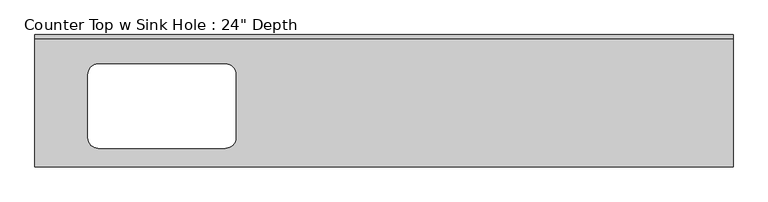
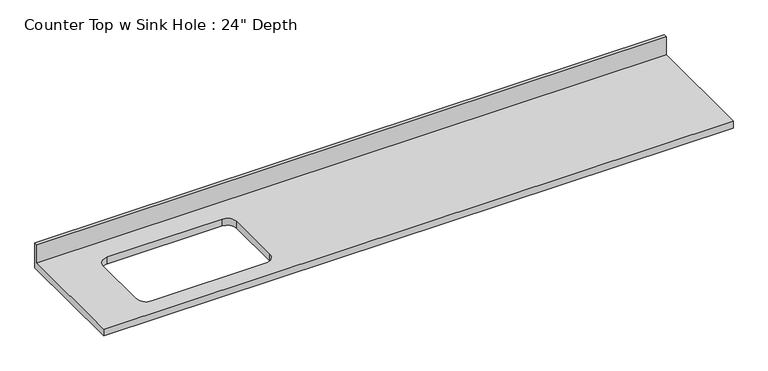
"""IFC4 building model written with IfcOpenShell, lengths in millimetres: furniture geometry."""

from ifc_helpers import new_model, si_unit, frame, origin, place, context, project, spatial, polyline, circle_curve, source, transform, mapped, element, save
from ifc_brep_helpers import plane_surface, revolved_surface, advanced_brep


def furniture_691b2c5f(model_context):
    return source(origin(), model_context, "Body", "AdvancedBrep", [
        advanced_brep(
        [(-1200.4622951, -635.0, 914.4), (2152.3377049, -635.0, 914.4), (2152.3377049, -19.05, 914.4), (-1200.4622951, -19.05, 914.4), (-895.6622951, -139.7, 914.4), (-286.0622951, -139.7, 914.4), (-235.2622951, -190.5, 914.4), (-235.2622951, -495.3, 914.4), (-286.0622951, -546.1, 914.4), (-895.6622951, -546.1, 914.4), (-946.4622951, -495.3, 914.4), (-946.4622951, -190.5, 914.4), (2152.3377049, 0.0, 876.3), (2152.3377049, -635.0, 876.3), (-1200.4622951, -635.0, 876.3), (-1200.4622951, 0.0, 876.3), (-286.0622951, -139.7, 876.3), (-895.6622951, -139.7, 876.3), (-946.4622951, -190.5, 876.3), (-946.4622951, -495.3, 876.3), (-895.6622951, -546.1, 876.3), (-286.0622951, -546.1, 876.3), (-235.2622951, -495.3, 876.3), (-235.2622951, -190.5, 876.3), (-1200.4622951, 0.0, 1016.0), (2152.3377049, 0.0, 1016.0), (-1200.4622951, -19.05, 1016.0), (2152.3377049, -19.05, 1016.0)],
        [
            (0, 1),
            (1, 2),
            (2, 3),
            (3, 0),
            (4, 5),
            (5, 6, circle_curve(frame((-286.0622951, -190.5, 914.4), z_axis=(0.0, 0.0, -1.0), x_axis=(1.0, 0.0, 0.0)), 50.8)),
            (6, 7),
            (7, 8, circle_curve(frame((-286.0622951, -495.3, 914.4), z_axis=(0.0, 0.0, -1.0), x_axis=(1.0, 0.0, 0.0)), 50.8)),
            (8, 9),
            (9, 10, circle_curve(frame((-895.6622951, -495.3, 914.4), z_axis=(0.0, 0.0, -1.0), x_axis=(1.0, 0.0, 0.0)), 50.8)),
            (10, 11),
            (11, 4, circle_curve(frame((-895.6622951, -190.5, 914.4), z_axis=(0.0, 0.0, -1.0), x_axis=(1.0, 0.0, 0.0)), 50.8)),
            (12, 13),
            (13, 14),
            (14, 15),
            (15, 12),
            (16, 17),
            (17, 18, circle_curve(frame((-895.6622951, -190.5, 876.3), z_axis=(0.0, 0.0, 1.0), x_axis=(1.0, 0.0, 0.0)), 50.8)),
            (18, 19),
            (19, 20, circle_curve(frame((-895.6622951, -495.3, 876.3), z_axis=(0.0, 0.0, 1.0), x_axis=(1.0, 0.0, 0.0)), 50.8)),
            (20, 21),
            (21, 22, circle_curve(frame((-286.0622951, -495.3, 876.3), z_axis=(0.0, 0.0, 1.0), x_axis=(1.0, 0.0, 0.0)), 50.8)),
            (22, 23),
            (23, 16, circle_curve(frame((-286.0622951, -190.5, 876.3), z_axis=(0.0, 0.0, 1.0), x_axis=(1.0, 0.0, 0.0)), 50.8)),
            (15, 24),
            (24, 25),
            (25, 12),
            (14, 0),
            (3, 26),
            (26, 24),
            (13, 1),
            (25, 27),
            (27, 2),
            (26, 27),
            (4, 17),
            (16, 5),
            (11, 18),
            (10, 19),
            (9, 20),
            (8, 21),
            (7, 22),
            (6, 23),
        ],
        [
            plane_surface(frame((-1200.4622951, 0.0, 914.4), z_axis=(0.0, 0.0, 1.0), x_axis=(-1.0, 0.0, 0.0))),
            plane_surface(frame((-1200.4622951, 0.0, 876.3), z_axis=(0.0, 0.0, -1.0), x_axis=(1.0, 0.0, 0.0))),
            plane_surface(frame((2152.3377049, 0.0, 914.4), z_axis=(0.0, 1.0, 0.0), x_axis=(0.0, 0.0, -1.0))),
            plane_surface(frame((-1200.4622951, 0.0, 914.4), z_axis=(-1.0, 0.0, 0.0), x_axis=(0.0, 0.0, -1.0))),
            plane_surface(frame((-1200.4622951, -635.0, 914.4), z_axis=(0.0, -1.0, 0.0), x_axis=(0.0, 0.0, -1.0))),
            plane_surface(frame((2152.3377049, -635.0, 914.4), z_axis=(1.0, 0.0, 0.0), x_axis=(0.0, 0.0, -1.0))),
            plane_surface(frame((-1200.4622951, 0.0, 1016.0), z_axis=(0.0, 0.0, 1.0), x_axis=(0.0, -1.0, 0.0))),
            plane_surface(frame((-1200.4622951, -19.05, 1016.0), z_axis=(0.0, -1.0, 0.0), x_axis=(0.0, 0.0, -1.0))),
            plane_surface(frame((-286.0622951, -139.7, 914.4), z_axis=(0.0, -1.0, 0.0), x_axis=(0.0, 0.0, -1.0))),
            revolved_surface(polyline([(-844.8622951000001, -190.5, 914.4), (-844.8622951000001, -190.5, 876.3)]), (-895.6622951, -190.5, 876.3), (0.0, 0.0, 1.0)),
            plane_surface(frame((-946.4622951, -190.5, 914.4), z_axis=(1.0, 0.0, 0.0), x_axis=(0.0, 0.0, -1.0))),
            revolved_surface(polyline([(-844.8622951000001, -495.3, 914.4), (-844.8622951000001, -495.3, 876.3)]), (-895.6622951, -495.3, 876.3), (0.0, 0.0, 1.0)),
            plane_surface(frame((-895.6622951, -546.1, 914.4), z_axis=(0.0, 1.0, 0.0), x_axis=(0.0, 0.0, -1.0))),
            revolved_surface(polyline([(-235.26229509999996, -495.3, 914.4), (-235.26229509999996, -495.3, 876.3)]), (-286.0622951, -495.3, 876.3), (0.0, 0.0, 1.0)),
            plane_surface(frame((-235.2622951, -495.3, 914.4), z_axis=(-1.0, 0.0, 0.0), x_axis=(0.0, 0.0, -1.0))),
            revolved_surface(polyline([(-235.26229509999996, -190.5, 914.4), (-235.26229509999996, -190.5, 876.3)]), (-286.0622951, -190.5, 876.3), (0.0, 0.0, 1.0)),
        ],
        [
            (0, [[1, 2, 3, 4], [5, 6, 7, 8, 9, 10, 11, 12]]),
            (1, [[13, 14, 15, 16], [17, 18, 19, 20, 21, 22, 23, 24]]),
            (2, [[-16, 25, 26, 27]]),
            (3, [[-15, 28, -4, 29, 30, -25]]),
            (4, [[-1, -28, -14, 31]]),
            (5, [[-13, -27, 32, 33, -2, -31]]),
            (6, [[-30, 34, -32, -26]]),
            (7, [[-34, -29, -3, -33]]),
            (8, [[35, -17, 36, -5]]),
            (9, [[-35, -12, 37, -18]]),
            (10, [[-37, -11, 38, -19]]),
            (11, [[-38, -10, 39, -20]]),
            (12, [[-39, -9, 40, -21]]),
            (13, [[-40, -8, 41, -22]]),
            (14, [[-41, -7, 42, -23]]),
            (15, [[-36, -24, -42, -6]]),
        ],
    ),
    ])


if __name__ == "__main__":
    model = new_model("IFC4")
    model_context = context("Model", 3, world=origin())
    ifc_project = project(units=[si_unit("LENGTHUNIT", "METRE", prefix="MILLI")], contexts=[model_context])
    site = spatial("IfcSite", under=ifc_project)
    building = spatial("IfcBuilding", under=site)
    placement = place(None, origin())
    furniture_shape = furniture_691b2c5f(model_context)
    element("IfcFurniture", 1, ObjectType="Counter Top w Sink Hole : 24\" Depth", at=placement, inside=building, context=model_context, shape_type="MappedRepresentation", body=[
        mapped(furniture_shape, transform((0.0, 0.0, 0.0), x_axis=(1.0, 0.0, 0.0), y_axis=(0.0, 1.0, 0.0), z_axis=(0.0, 0.0, 1.0))),
    ])
    save(model, "model.ifc")

# Revit data of these elements
# Type "Counter Top w Sink Hole : 24\" Depth"
#   Assembly Code = "C1030400"
#   Counter Thickness = 0' - 1 1/2"
#   Depth = 2' - 1"
#   Height = 3' - 0"
#   Length [instance default] = 8' - 0"
#   Sink Location [instance default] = 2' - 0"
#   Sink Location To Wall [instance default] = 0' - 6"
#   Sink Opening Depth [instance default] = 1' - 3"
#   Sink Opening Width [instance default] = 2' - 3"
#   Counter Top Material = none
#   Default Elevation = 0
# Element 1 (IfcFurniture, "Counter Top w Sink Hole : 24\" Depth")
#   Length = 11' - 0"
#   Materials on its faces: "Counter Top"
# Materials
#   "Counter Top": class "Wood", colour RGB 226 177 128, transparency 0
